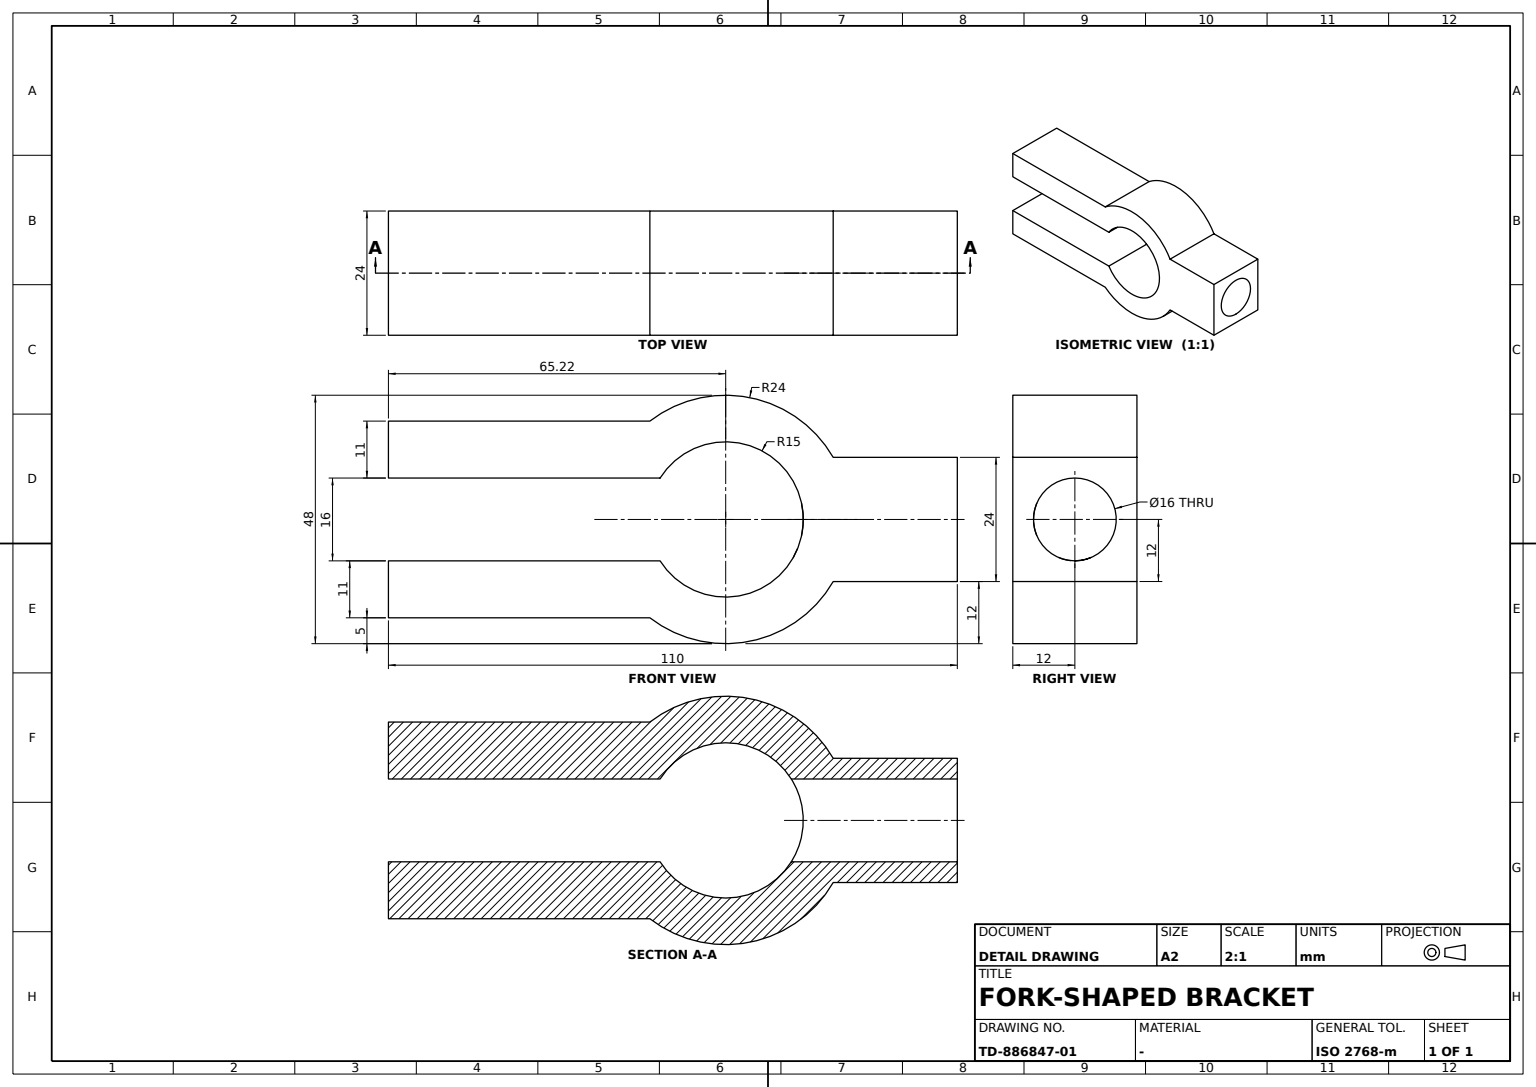
CATIA V5 part; units mm, degrees
sketch "Sketch1" plane through (0, 0, 0) normal (0, 1, 0) x (-1, 0, 0)
  arc A0 (14.6629, 19) -> (-20.7846, 12) centre (0, 0) ccw
  line L0 (14.6629, 19) -> (65.2154, 19)
  line L1 (65.2154, 19) -> (65.2154, 8)
  point P0 (65.2154, 8)
  point P1 (14.6629, -19)
  line L2 (14.6629, -19) -> (65.2154, -19)
  line L3 (65.2154, -19) -> (65.2154, -8)
  point P2 (65.2154, -8)
  point P3 (-44.7846, 12)
  line L4 (-44.7846, 12) -> (-44.7846, -12)
  point P4 (-44.7846, -12)
  arc A1 (-20.7846, -12) -> (14.6629, -19) centre (0, 0) ccw
  point P5 (-44.7846, 12)
  line L5 (-44.7846, 12) -> (-20.7846, 12)
  point P6 (-44.7846, -12)
  line L6 (-44.7846, -12) -> (-20.7846, -12)
  line L7 (65.2154, 8) -> (12.6886, 8)
  line L8 (65.2154, -8) -> (12.6886, -8)
  arc A2 (12.6886, 8) -> (12.6886, -8) centre (0, 0) ccw
  point P7 (9, -12)
  dimension "radius A0" = 24
  dimension "length L3" = 11
  dimension "length L1" = 11
  dimension "distance P4 L3" = 110
  dimension "distance P3 L1" = 110
  dimension "distance P0 P2" = 16
  dimension "length L4" = 24
  dimension "length L5" = 24
  dimension "radius A2" = 15
  constraint horizontal L0 x-axis
  constraint horizontal L2 x-axis
  constraint horizontal L5 x-axis
  constraint horizontal L6 x-axis
  constraint horizontal L7 x-axis
  constraint horizontal L8 x-axis
  constraint vertical L1 y-axis
  constraint vertical L3 y-axis
  constraint vertical L4 y-axis
  constraint coincidence P1 A0
  constraint coincidence A0 A1
  constraint coincidence P5 L4
  constraint coincidence P5 P3
  constraint coincidence P6 P4
  constraint coincidence A2 P7
  constraint coincidence P7 L6
  constraint symmetry L5 L6 x-axis
  constraint symmetry L0 L2 x-axis
extrude "Pad1" add sketch "Sketch1" along normal mid plane 24
sketch "Sketch2" plane through (44.7846, 0, 0) normal (1, 0, 0) x (0, 1, 0)
  circle A0 centre (0, 0) radius 8
  dimension "radius A0" = 8
extrude "Pocket1" cut sketch "Sketch2" against normal up to next
